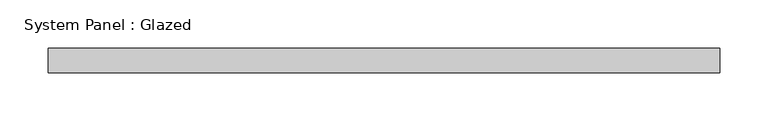
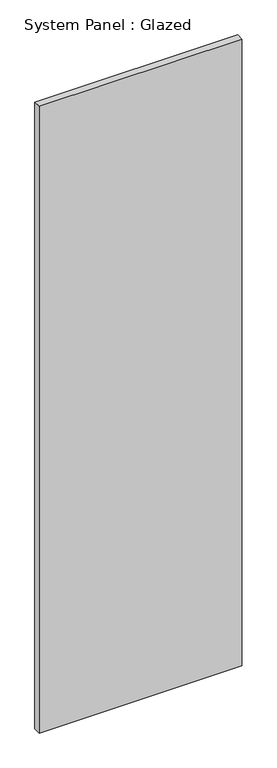
"""IFC4 building model written with IfcOpenShell, lengths in millimetres: plate geometry, System Panel : Glazed."""

from ifc_helpers import new_model, si_unit, origin, origin_with_axes, place, context, project, spatial, polyline, outline, extrude, source, transform, mapped, element, save


def system_panel_glazed_9b1662f5(model_context):
    return source(origin(), model_context, "Body", "SweptSolid", [
        extrude(outline(polyline([(349.25, 19.05), (-349.25, 19.05), (-349.25, 44.45), (349.25, 44.45), (349.25, 19.05)])), origin_with_axes(), (0.0, 0.0, 1.0), 2284.5809615),
    ])


if __name__ == "__main__":
    model = new_model("IFC4")
    model_context = context("Model", 3, world=origin())
    ifc_project = project(units=[si_unit("LENGTHUNIT", "METRE", prefix="MILLI")], contexts=[model_context])
    site = spatial("IfcSite", under=ifc_project)
    building = spatial("IfcBuilding", under=site)
    placement = place(None, origin())
    system_panel_glazed_shape = system_panel_glazed_9b1662f5(model_context)
    element("IfcPlate", 1, ObjectType="System Panel : Glazed", at=placement, inside=building, context=model_context, shape_type="MappedRepresentation", body=[
        mapped(system_panel_glazed_shape, transform((0.0, 0.0, 0.0), x_axis=(1.0, 0.0, 0.0), y_axis=(0.0, 1.0, 0.0), z_axis=(0.0, 0.0, 1.0))),
    ])
    save(model, "model.ifc")

# Revit data of these elements
# Type "System Panel : Glazed"
#   Construction Type Id = "GSP4R"
#   Analytic Construction = "1/8 in Pilkington single glazing"
#   Visual Light Transmittance = 0.9
#   Solar Heat Gain Coefficient = 0.86
#   Heat Transfer Coefficient (U) = 1.18115 BTU/(h·ft²·°F)
#   Define Thermal Properties by = 1
# Element 1 (IfcPlate, "System Panel : Glazed")
#   Materials on its faces: "Glass"
# Materials
#   "Glass": class "Glass", colour RGB 0 128 192, transparency 0.75, Description = "Soda Lime Glass", Cost = 0
